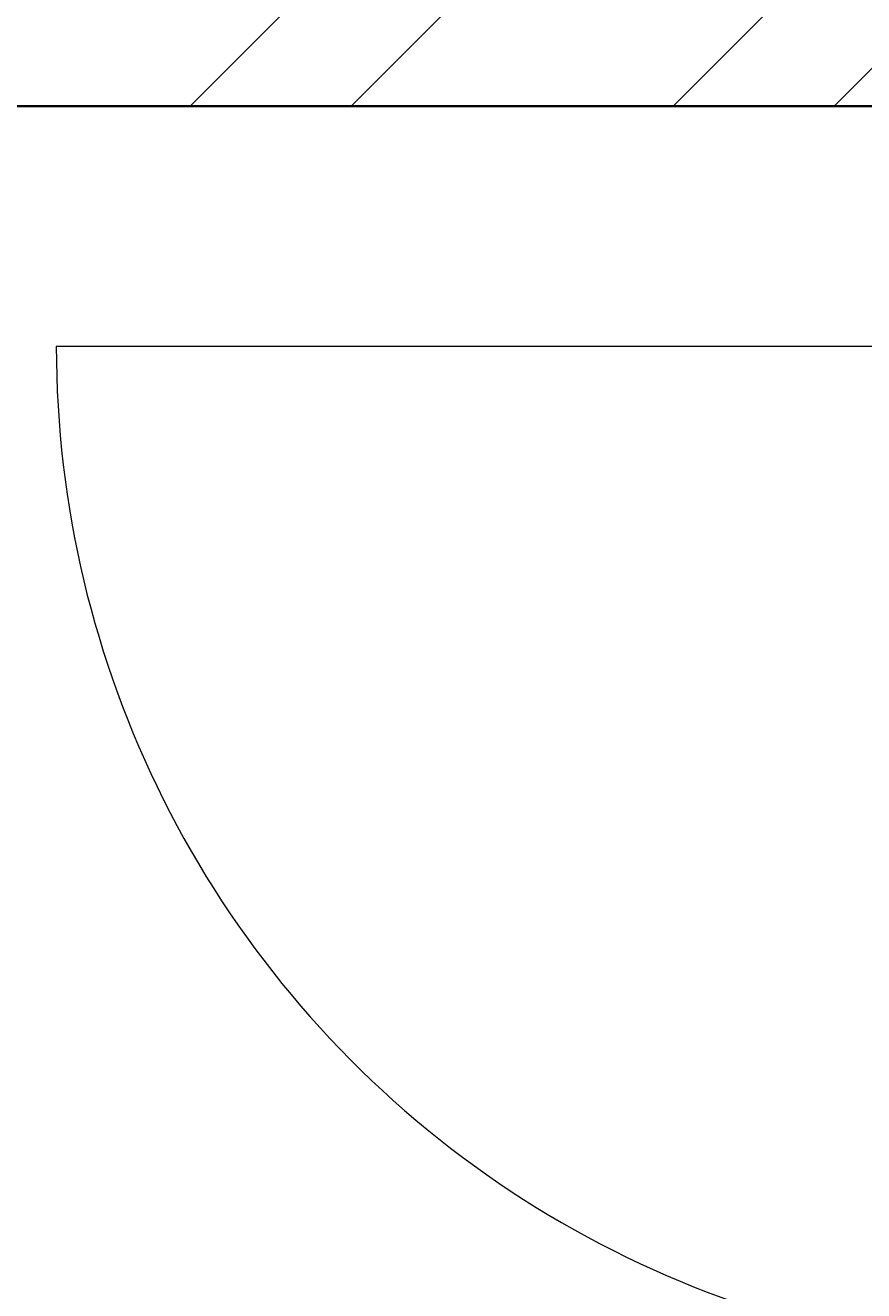
# Model space of a CAD drawing. Units: inches. Extents: x 1962 to 2771, y 1245 to 2660.
# Tile 58 of 114: x 2200 to 2224, y 2145 to 2180. Entities that reach past the tile are written whole.
import ezdxf

# ---------------------------------------------------------------- set-up
doc = ezdxf.new("R2010")
doc.units = ezdxf.units.IN
for name, color, linetype, lineweight in [('A-ANNO-DIMS', 2, 'Continuous', 18), ('A-DOOR', 3, 'Continuous', 18), ('A-WALL', 7, 'Continuous', 35), ('A-WALL-PATT', 252, 'Continuous', 13)]:
    doc.layers.add(name, color=color, linetype=linetype, lineweight=lineweight)
doc.styles.get("Standard").update_dxf_attribs({"font": 'arial.ttf'})
doc.dimstyles.get("Standard").update_dxf_attribs({"dimtxt": 0.18, "dimasz": 0.18, "dimexe": 0.18, "dimexo": 0.0625, "dimgap": 0.09, "dimtad": 0, "dimtih": 1, "dimtoh": 1, "dimdec": 4, "dimzin": 0, "dimdsep": 46, "dimtxsty": 'Standard', "dimcen": 0.09, "dimadec": 0, "dimazin": 0, "dimtfac": 1, "dimtdec": 4, "dimtofl": 0, "dimtmove": 0, "dimatfit": 3, "dimfxl": 1, "dimtolj": 1, "dimtzin": 0, "dimarcsym": 0})

# ---------------------------------------------------------------- blocks, each defined once
blk = doc.blocks.new('*D40')
at = {"layer": 'A-ANNO-DIMS', "color": 0, "lineweight": -2, "transparency": 16777216}
for p, q in [((2072.02, 2033.906), (2072.02, 2583.474)), ((2072.2, 2583.294), (2366.02, 2583.294)), ((2660.627, 2583.294), (2366.808, 2583.294)), ((2660.807, 2524.406), (2660.807, 2583.474))]:
    blk.add_line(p, q, dxfattribs=at)
at = {"layer": 'A-ANNO-DIMS', "color": 0, "transparency": 16777216}
for points in [[(2072.2, 2583.324), (2072.2, 2583.264), (2072.02, 2583.294)], [(2660.627, 2583.324), (2660.627, 2583.264), (2660.807, 2583.294)]]:
    blk.add_solid(points, dxfattribs=at)
at = {"layer": 'Defpoints', "color": 0, "transparency": 16777216}
for p in [(2660.807, 2583.294), (2660.807, 2524.344), (2072.02, 2033.844)]:
    blk.add_point(p, dxfattribs=at)
at = {"layer": 'A-ANNO-DIMS', "color": 0, "transparency": 16777216, "insert": (2366.414, 2583.294), "char_height": 0.18, "attachment_point": 5}
blk.add_mtext('\\A1;588.8', dxfattribs=at)

msp = doc.modelspace()

# ---------------------------------------------------------------- hatches: boundary and pattern name
at = {"layer": 'A-WALL-PATT'}
h = msp.add_hatch(dxfattribs=at)
h.set_pattern_fill('ANSI32', color=256)
h.paths.add_polyline_path([(2090.8074, 2467.3437), (2141.6481, 2467.3437), (2141.6481, 2469.5937), (2141.6481, 2471.8437), (2086.3074, 2471.8437), (2086.3074, 2422.5333), (2090.8074, 2422.5333)])
h.paths.add_polyline_path([(2282.7664, 2471.8437), (2204.8982, 2471.8437), (2204.8982, 2467.3437), (2234.8074, 2467.3437), (2234.8074, 2311.3437), (2228.7492, 2311.3437), (2228.7492, 2306.8437), (2234.8074, 2306.8437), (2331.9227, 2306.8437), (2331.9227, 2309.0937), (2331.9227, 2311.3437), (2239.3074, 2311.3437), (2239.3074, 2467.3437), (2282.7664, 2467.3437), (2282.7664, 2469.5937)])
h.paths.add_polyline_path([(2471.4531, 2519.8437), (2552.011, 2519.8437), (2564.3996, 2519.8437), (2564.3996, 2511.1389), (2568.8996, 2511.1389), (2568.8996, 2524.3437), (2466.9531, 2524.3437), (2466.9531, 2471.8437), (2450.0749, 2471.8437), (2446.4672, 2471.8437), (2446.4672, 2467.3437), (2450.0749, 2467.3437), (2475.9988, 2467.3437), (2475.9988, 2469.5937), (2475.9988, 2471.8437), (2471.4531, 2471.8437)])
h.paths.add_polyline_path([(2575.2231, 2469.5937), (2575.2231, 2471.8437), (2568.8996, 2471.8437), (2568.8996, 2487.1389), (2564.3996, 2487.1389), (2564.3996, 2471.8437), (2556.511, 2471.8437), (2499.2904, 2471.8437), (2499.2904, 2467.3437), (2507.8074, 2467.3437), (2507.8074, 2311.3437), (2414.863, 2311.3437), (2414.863, 2306.8437), (2512.3074, 2306.8437), (2517.0114, 2306.8437), (2517.0114, 2309.0937), (2517.0114, 2311.3437), (2512.3074, 2311.3437), (2512.3074, 2467.3437), (2575.2231, 2467.3437)])
h.paths.add_polyline_path([(2660.8074, 2471.8437), (2600.9602, 2471.8437), (2600.9602, 2467.3437), (2656.3074, 2467.3437), (2656.3074, 2432.5704), (2660.8074, 2432.5704)])
h.paths.add_polyline_path([(2660.8074, 2372.5704), (2656.3074, 2372.5704), (2656.3074, 2311.3437), (2600.276, 2311.3437), (2600.276, 2309.0937), (2600.276, 2306.8437), (2656.3074, 2306.8437), (2656.3074, 2296.2593), (2660.8074, 2296.2593)])
h.paths.add_polyline_path([(2572.3074, 2306.8437), (2577.1385, 2306.8437), (2577.1385, 2311.3437), (2551.082, 2311.3437), (2551.082, 2306.8437), (2567.8074, 2306.8437), (2567.8074, 2258.8437), (2540.0574, 2258.8437), (2540.0574, 2256.5937), (2540.0574, 2254.3437), (2567.8074, 2254.3437), (2656.3074, 2254.3437), (2656.3074, 2236.9085), (2660.8074, 2236.9085), (2660.8074, 2272.2593), (2656.3074, 2272.2593), (2656.3074, 2258.8437), (2572.3074, 2258.8437)])
h.paths.add_polyline_path([(2512.3074, 2254.3437), (2518.8716, 2254.3437), (2518.8716, 2256.5937), (2518.8716, 2258.8437), (2507.8074, 2258.8437), (2507.8074, 2177.8437), (2567.8074, 2177.8437), (2567.8074, 2172.9628), (2572.3074, 2172.9628), (2572.3074, 2177.8437), (2656.3074, 2177.8437), (2656.3074, 2166.4846), (2660.8074, 2166.4846), (2660.8074, 2200.9085), (2656.3074, 2200.9085), (2656.3074, 2182.3437), (2512.3074, 2182.3437)])
h.paths.add_polyline_path([(2656.3074, 2129.8437), (2572.3074, 2129.8437), (2572.3074, 2150.3044), (2570.0574, 2150.3044), (2567.8074, 2150.3044), (2567.8074, 2129.8437), (2507.8074, 2129.8437), (2507.8074, 2116.3027), (2510.0574, 2116.3027), (2512.3074, 2116.3027), (2512.3074, 2125.3437), (2567.8074, 2125.3437), (2572.3074, 2125.3437), (2656.3074, 2125.3437)])
h.paths.add_polyline_path([(2090.8074, 2362.5333), (2086.3074, 2362.5333), (2086.3074, 2298.6242), (2090.8074, 2298.6242), (2090.8074, 2306.8437), (2174.8074, 2306.8437), (2174.8074, 2286.4178), (2179.3074, 2286.4178), (2179.3074, 2306.8437), (2192.8641, 2306.8437), (2192.8641, 2309.0937), (2192.8641, 2311.3437), (2090.8074, 2311.3437)])
h.paths.add_polyline_path([(2209.156, 2258.8437), (2179.3074, 2258.8437), (2179.3074, 2263.2236), (2177.0574, 2263.2236), (2174.8074, 2263.2236), (2174.8074, 2258.8437), (2090.8074, 2258.8437), (2090.8074, 2274.6242), (2086.3074, 2274.6242), (2086.3074, 2238.2967), (2088.5574, 2238.2967), (2090.8074, 2238.2967), (2090.8074, 2254.3437), (2209.156, 2254.3437)])
h.paths.add_polyline_path([(2090.8074, 2177.8437), (2234.8074, 2177.8437), (2234.8074, 2173.1428), (2239.3074, 2173.1428), (2239.3074, 2258.8437), (2230.8442, 2258.8437), (2230.8442, 2256.5937), (2230.8442, 2254.3437), (2234.8074, 2254.3437), (2234.8074, 2182.3437), (2090.8074, 2182.3437), (2090.8074, 2202.2967), (2086.3074, 2202.2967), (2086.3074, 2140.0389), (2090.8074, 2140.0389)])
h.paths.add_polyline_path([(2090.8074, 2080.0389), (2086.3074, 2080.0389), (2086.3074, 2033.8437), (2090.8074, 2033.8437)], flags=17)
h.paths.add_polyline_path([(2244.9405, 2033.8437), (2239.3074, 2033.8437), (2239.3074, 2142.0665), (2237.2592, 2142.0665), (2234.8074, 2142.0665), (2234.8074, 2033.8437), (2090.8074, 2033.8437), (2076.5204, 2033.8437), (2072.0204, 2033.8437), (2072.0204, 2000.4493), (2076.5204, 2000.4493), (2076.5204, 2029.3437), (2090.8074, 2029.3437), (2244.9405, 2029.3437), (2244.9405, 2031.5937)])
h.paths.add_polyline_path([(2234.8074, 1933.3437), (2076.5204, 1933.3437), (2076.5204, 1952.4493), (2074.2704, 1952.4493), (2072.0204, 1952.4493), (2072.0204, 1933.3437), (2072.0204, 1928.8437), (2234.8074, 1928.8437)])
h.paths.add_polyline_path([(2090.8074, 1928.8437), (2086.3074, 1928.8437), (2086.3074, 1906.5013), (2090.8074, 1906.5013)])
h.paths.add_polyline_path([(2090.8074, 1846.5013), (2086.3074, 1846.5013), (2086.3074, 1769.9917), (2088.5574, 1769.9917), (2090.8074, 1769.9917), (2090.8074, 1780.3437), (2234.8074, 1780.3437), (2234.8074, 1708.3437), (2230.3764, 1708.3437), (2230.3764, 1703.8437), (2239.3074, 1703.8437), (2239.3074, 1792.6669), (2237.0574, 1792.6669), (2234.8074, 1792.6669), (2234.8074, 1784.8437), (2090.8074, 1784.8437)])
h.paths.add_polyline_path([(2239.3074, 1928.8437), (2244.9405, 1928.8437), (2244.9405, 1931.0937), (2244.9405, 1933.3437), (2234.8074, 1933.3437), (2234.8074, 1928.8437), (2234.8074, 1825.5949), (2239.3074, 1825.5949)])
h.paths.add_polyline_path([(2148.0425, 1649.0937), (2148.0425, 1651.3437), (2090.8074, 1651.3437), (2090.8074, 1646.8437), (2148.0425, 1646.8437)], flags=0)
h.paths.add_polyline_path([(2207.5601, 1708.3437), (2090.8074, 1708.3437), (2090.8074, 1703.8437), (2174.8074, 1703.8437), (2174.8074, 1651.3437), (2170.4457, 1651.3437), (2170.4457, 1646.8437), (2195.9924, 1646.8437), (2195.9924, 1649.0937), (2195.9924, 1651.3437), (2179.3074, 1651.3437), (2179.3074, 1703.8437), (2207.5601, 1703.8437), (2207.5601, 1706.0937)])
h.paths.add_polyline_path([(2090.8074, 1733.9917), (2086.3074, 1733.9917), (2086.3074, 1696.1032), (2088.5574, 1696.1032), (2090.8074, 1696.1032)])
h.paths.add_polyline_path([(2090.8074, 1672.1032), (2086.3074, 1672.1032), (2086.3074, 1600.3335), (2090.8074, 1600.3335)])
h.paths.add_polyline_path([(2090.8074, 1540.3335), (2086.3074, 1540.3335), (2086.3074, 1486.3437), (2139.6766, 1486.3437), (2139.6766, 1490.8437), (2090.8074, 1490.8437)])
h.paths.add_polyline_path([(2302.3876, 1490.8437), (2239.3074, 1490.8437), (2239.3074, 1646.8437), (2335.9994, 1646.8437), (2335.9994, 1651.3437), (2229.884, 1651.3437), (2229.884, 1646.8437), (2234.8074, 1646.8437), (2234.8074, 1490.8437), (2202.7103, 1490.8437), (2202.7103, 1488.5937), (2202.7103, 1486.3437), (2275.0699, 1486.3437), (2275.0699, 1475.772), (2279.5699, 1475.772), (2279.5699, 1486.3437), (2302.3876, 1486.3437)])
h.paths.add_polyline_path([(2279.5699, 1451.772), (2275.0699, 1451.772), (2275.0699, 1438.3437), (2174.8074, 1438.3437), (2174.8074, 1486.3437), (2179.7922, 1486.3437), (2179.7922, 1490.8437), (2163.3585, 1490.8437), (2163.3585, 1488.5937), (2163.3585, 1486.3437), (2170.3074, 1486.3437), (2170.3074, 1433.8437), (2279.5699, 1433.8437)])
h.paths.add_polyline_path([(2427.2363, 1490.8437), (2375.8074, 1490.8437), (2375.8074, 1646.8437), (2381.6401, 1646.8437), (2381.6401, 1651.3437), (2365.887, 1651.3437), (2365.887, 1649.0937), (2365.887, 1646.8437), (2371.3074, 1646.8437), (2371.3074, 1490.8437), (2327.5627, 1490.8437), (2327.5627, 1488.5937), (2327.5627, 1486.3437), (2371.3074, 1486.3437), (2371.3074, 1433.8437), (2375.8074, 1433.8437), (2375.8074, 1486.3437), (2427.2363, 1486.3437)])
h.paths.add_polyline_path([(2512.3074, 1646.8437), (2519.4351, 1646.8437), (2519.4351, 1649.0937), (2519.4351, 1651.3437), (2507.8074, 1651.3437), (2416.0063, 1651.3437), (2416.0063, 1649.0937), (2416.0063, 1646.8437), (2507.8074, 1646.8437), (2507.8074, 1490.8437), (2497.0532, 1490.8437), (2497.0532, 1488.5937), (2497.0532, 1486.3437), (2574.9344, 1486.3437), (2574.9344, 1476.0181), (2579.4344, 1476.0181), (2579.4344, 1486.3437), (2584.4872, 1486.3437), (2584.3074, 1490.8437), (2512.3074, 1490.8437)])
h.paths.add_polyline_path([(2470.5091, 1486.3437), (2473.9767, 1486.3437), (2473.9767, 1490.8437), (2449.6605, 1490.8437), (2449.6605, 1488.5937), (2449.6605, 1486.3437), (2466.0091, 1486.3437), (2466.0091, 1433.8437), (2470.5091, 1433.8437), (2579.4344, 1433.8437), (2579.4344, 1452.0181), (2574.9344, 1452.0181), (2574.9344, 1438.3437), (2554.5091, 1438.3437), (2470.5091, 1438.3437)])
h.paths.add_polyline_path([(2656.3074, 1490.8437), (2611.86, 1490.8437), (2611.86, 1486.3437), (2656.3074, 1486.3437)])
h.paths.add_polyline_path([(2660.8074, 1532.7007), (2658.5574, 1532.7007), (2656.3074, 1532.7007), (2656.3074, 1486.3437), (2660.8074, 1486.3437)])
h.paths.add_polyline_path([(2660.8074, 1664.9663), (2656.3074, 1664.9663), (2656.3074, 1651.3437), (2602.2313, 1651.3437), (2602.2313, 1646.8437), (2656.3074, 1646.8437), (2656.3074, 1592.7007), (2660.8074, 1592.7007)])
h.paths.add_polyline_path([(2660.8074, 1724.5221), (2656.3074, 1724.5221), (2656.3074, 1703.8437), (2542.4725, 1703.8437), (2542.4725, 1699.3437), (2567.8074, 1699.3437), (2567.8074, 1651.3437), (2552.7766, 1651.3437), (2552.7766, 1649.0937), (2552.7766, 1646.8437), (2577.2878, 1646.8437), (2577.2878, 1649.0937), (2577.2878, 1651.3437), (2572.3074, 1651.3437), (2572.3074, 1699.3437), (2656.3074, 1699.3437), (2656.3074, 1688.9663), (2660.8074, 1688.9663)])
h.paths.add_polyline_path([(2660.8074, 1880.6524), (2656.3074, 1880.6524), (2656.3074, 1832.8437), (2512.3074, 1832.8437), (2512.3074, 1837.8959), (2507.8074, 1837.8959), (2507.8074, 1828.3437), (2567.8074, 1828.3437), (2567.8074, 1804.3437), (2572.3074, 1804.3437), (2572.3074, 1828.3437), (2656.3074, 1828.3437), (2656.3074, 1818.6778), (2660.8074, 1818.6778)])
h.paths.add_polyline_path([(2660.8074, 1794.6778), (2656.3074, 1794.6778), (2656.3074, 1780.3437), (2572.3074, 1780.3437), (2572.3074, 1783.0303), (2570.0574, 1783.0303), (2567.8074, 1783.0303), (2567.8074, 1780.3437), (2507.8074, 1780.3437), (2507.8074, 1699.3437), (2517.8858, 1699.3437), (2517.8858, 1701.5937), (2517.8858, 1703.8437), (2512.3074, 1703.8437), (2512.3074, 1775.8437), (2656.3074, 1775.8437), (2656.3074, 1760.5221), (2660.8074, 1760.5221)])
h.paths.add_polyline_path([(2660.8074, 1981.3437), (2660.8074, 2020.2808), (2658.5574, 2020.2808), (2656.3074, 2020.2808), (2656.3074, 1981.3437), (2512.3074, 1981.3437), (2512.3074, 2086.6996), (2507.8074, 2086.6996), (2507.8074, 1981.3437), (2375.8074, 1981.3437), (2375.8074, 1986.8505), (2373.5574, 1986.8505), (2371.3074, 1986.8505), (2371.3074, 1973.2607), (2375.8074, 1973.2607), (2375.8074, 1976.8437), (2507.8074, 1976.8437), (2507.8074, 1865.4281), (2510.0574, 1865.4281), (2512.3074, 1865.4281), (2512.3074, 1976.8437), (2660.8074, 1976.8437)])
h.paths.add_polyline_path([(2375.8074, 1940.297), (2373.5574, 1940.297), (2371.3074, 1940.297), (2371.3074, 1933.3437), (2278.4434, 1933.3437), (2278.4434, 1928.8437), (2371.3074, 1928.8437), (2371.3074, 1651.3437), (2375.8074, 1651.3437)])
h.paths.add_polyline_path([(2660.8074, 1976.8437), (2656.3074, 1976.8437), (2656.3074, 1940.6524), (2660.8074, 1940.6524)], flags=17)
h.paths.add_polyline_path([(2660.8074, 2142.4846), (2656.3074, 2142.4846), (2656.3074, 2080.2808), (2660.8074, 2080.2808)])
h.paths.add_polyline_path([(2381.4189, 2311.3437), (2375.8074, 2311.3437), (2375.8074, 2467.3437), (2424.7242, 2467.3437), (2424.7242, 2469.5937), (2424.7242, 2471.8437), (2375.8074, 2471.8437), (2375.8074, 2524.3437), (2371.3074, 2524.3437), (2371.3074, 2471.8437), (2307.2097, 2471.8437), (2307.2097, 2467.3437), (2371.3074, 2467.3437), (2371.3074, 2311.3437), (2366.8901, 2311.3437), (2366.8901, 2306.8437), (2371.3074, 2306.8437), (2371.3074, 2033.8437), (2279.6589, 2033.8437), (2279.6589, 2029.3437), (2371.3074, 2029.3437), (2371.3074, 2014.2598), (2375.8074, 2014.2598), (2375.8074, 2306.8437), (2381.4189, 2306.8437)])
h.paths.add_polyline_path([(2263.3074, 2524.3437), (2170.3074, 2524.3437), (2170.3074, 2519.8437), (2170.3074, 2471.8437), (2165.0312, 2471.8437), (2165.0312, 2467.3437), (2179.6721, 2467.3437), (2179.6721, 2469.5161), (2179.6721, 2471.8437), (2174.8074, 2471.8437), (2174.8074, 2519.8437), (2258.8074, 2519.8437), (2258.8074, 2511.6436), (2263.3074, 2511.6436)])
h.paths.add_polyline_path([(2245.0232, 1361.4123), (2492.9468, 1361.4123), (2492.9468, 1398.505), (2245.0232, 1398.505)], flags=9)
h.paths.add_polyline_path([(2388.1434, 2086.6936), (2425.0704, 2086.6936), (2425.0704, 2105.3509), (2388.1434, 2105.3509)], flags=9)
h.paths.add_polyline_path([(2404.922, 2242.6744), (2445.7337, 2242.6744), (2445.7337, 2261.3318), (2404.922, 2261.3318)], flags=9)
h.paths.add_polyline_path([(2269.4107, 2156.7935), (2306.3378, 2156.7935), (2306.3378, 2175.4508), (2269.4107, 2175.4508)], flags=9)
h.paths.add_polyline_path([(2269.3277, 2233.4343), (2306.2547, 2233.4343), (2306.2547, 2252.0917), (2269.3277, 2252.0917)], flags=9)
h.paths.add_polyline_path([(2431.6052, 2320.6922), (2470.4456, 2320.6922), (2470.4456, 2339.3495), (2431.6052, 2339.3495)], flags=25)
h.paths.add_polyline_path([(2249.6902, 2315.7608), (2288.5306, 2315.7608), (2288.5306, 2334.4182), (2249.6902, 2334.4182)], flags=25)
h.paths.add_polyline_path([(2096.9301, 2314.3181), (2135.7704, 2314.3181), (2135.7704, 2332.9755), (2096.9301, 2332.9755)], flags=25)
h.paths.add_polyline_path([(2134.3475, 2285.7089), (2161.4655, 2285.7089), (2161.4655, 2304.3662), (2134.3475, 2304.3662)], flags=9)
h.paths.add_polyline_path([(2126.5155, 2209.4076), (2159.9227, 2209.4076), (2159.9227, 2228.065), (2126.5155, 2228.065)], flags=25)
h.paths.add_polyline_path([(2110.5753, 2141.5299), (2149.4157, 2141.5299), (2149.4157, 2160.1872), (2110.5753, 2160.1872)], flags=25)
h.paths.add_polyline_path([(2249.8618, 1968.3317), (2286.3966, 1968.3317), (2286.3966, 1986.989), (2249.8618, 1986.989)], flags=9)
h.paths.add_polyline_path([(2395.9507, 1777.0051), (2436.7624, 1777.0051), (2436.7624, 1795.6625), (2395.9507, 1795.6625)], flags=9)
h.paths.add_polyline_path([(2398.5259, 1888.5651), (2435.0062, 1888.5651), (2435.0062, 1907.2224), (2398.5259, 1907.2224)], flags=25)
h.paths.add_polyline_path([(2259.3506, 1728.3559), (2296.2776, 1728.3559), (2296.2776, 1747.0132), (2259.3506, 1747.0132)], flags=9)
h.paths.add_polyline_path([(2271.3698, 1845.268), (2308.2968, 1845.268), (2308.2968, 1863.9253), (2271.3698, 1863.9253)], flags=9)
h.paths.add_polyline_path([(2120.9355, 1786.3027), (2159.7759, 1786.3027), (2159.7759, 1804.9601), (2120.9355, 1804.9601)], flags=25)
h.paths.add_polyline_path([(2121.3164, 1732.1043), (2154.7236, 1732.1043), (2154.7236, 1750.7616), (2121.3164, 1750.7616)], flags=25)
h.paths.add_polyline_path([(2118.3706, 1678.8997), (2147.5282, 1678.8997), (2147.5282, 1697.557), (2118.3706, 1697.557)], flags=25)
h.paths.add_polyline_path([(2385.9227, 1493.557), (2424.763, 1493.557), (2424.763, 1512.2143), (2385.9227, 1512.2143)], flags=25)
h.paths.add_polyline_path([(2248.7058, 1500.0256), (2287.5462, 1500.0256), (2287.5462, 1518.6829), (2248.7058, 1518.6829)], flags=25)
h.paths.add_polyline_path([(2104.1669, 1617.3771), (2143.0073, 1617.3771), (2143.0073, 1636.0344), (2104.1669, 1636.0344)], flags=9)
h.paths.add_polyline_path([(2096.0714, 1447.8824), (2137.3845, 1447.8824), (2137.3845, 1458.1859), (2096.0714, 1458.1859)], flags=9)
h.paths.add_polyline_path([(2180.6114, 1440.325), (2209.7689, 1440.325), (2209.7689, 1458.9823), (2180.6114, 1458.9823)], flags=25)
h.paths.add_polyline_path([(2316.1698, 1447.9637), (2357.4829, 1447.9637), (2357.4829, 1458.2673), (2316.1698, 1458.2673)], flags=9)
h.paths.add_polyline_path([(2397.6187, 1447.9637), (2438.9318, 1447.9637), (2438.9318, 1458.2673), (2397.6187, 1458.2673)], flags=9)
h.paths.add_polyline_path([(2473.0778, 1439.5953), (2502.2354, 1439.5953), (2502.2354, 1458.2527), (2473.0778, 1458.2527)], flags=25)
h.paths.add_polyline_path([(2589.7027, 1447.8819), (2631.0158, 1447.8819), (2631.0158, 1458.1855), (2589.7027, 1458.1855)], flags=9)
h.paths.add_polyline_path([(2522.4009, 1497.5285), (2561.2413, 1497.5285), (2561.2413, 1516.1859), (2522.4009, 1516.1859)], flags=25)
h.paths.add_polyline_path([(2579.6565, 1671.3482), (2608.8141, 1671.3482), (2608.8141, 1690.0056), (2579.6565, 1690.0056)], flags=25)
h.paths.add_polyline_path([(2544.7038, 1725.5064), (2578.1111, 1725.5064), (2578.1111, 1744.1637), (2544.7038, 1744.1637)], flags=25)
h.paths.add_polyline_path([(2578.1191, 1807.472), (2607.2766, 1807.472), (2607.2766, 1826.1293), (2578.1191, 1826.1293)], flags=25)
h.paths.add_polyline_path([(2595.0614, 1835.1839), (2633.9018, 1835.1839), (2633.9018, 1853.8413), (2595.0614, 1853.8413)], flags=25)
h.paths.add_polyline_path([(2567.0097, 2097.7035), (2605.8501, 2097.7035), (2605.8501, 2116.3609), (2567.0097, 2116.3609)], flags=9)
h.paths.add_polyline_path([(2586.644, 2134.6454), (2615.8015, 2134.6454), (2615.8015, 2153.3027), (2586.644, 2153.3027)], flags=9)
h.paths.add_polyline_path([(2544.6185, 2212.6783), (2578.0258, 2212.6783), (2578.0258, 2231.3356), (2544.6185, 2231.3356)], flags=25)
h.paths.add_polyline_path([(2577.0273, 2256.9023), (2606.1849, 2256.9023), (2606.1849, 2275.5597), (2577.0273, 2275.5597)], flags=24)
h.paths.add_polyline_path([(2605.2683, 2315.2821), (2644.1087, 2315.2821), (2644.1087, 2333.9395), (2605.2683, 2333.9395)], flags=25)
h.paths.add_polyline_path([(2583.1244, 2496.1815), (2624.4375, 2496.1815), (2624.4375, 2506.4851), (2583.1244, 2506.4851)], flags=9)
h.paths.add_polyline_path([(2474.761, 2497.0823), (2503.9185, 2497.0823), (2503.9185, 2515.7397), (2474.761, 2515.7397)], flags=25)
h.paths.add_polyline_path([(2387.5787, 2494.2563), (2428.902, 2494.2563), (2428.902, 2504.5598), (2387.5787, 2504.5598)], flags=9)
h.paths.add_polyline_path([(2300.1657, 2500.1564), (2341.4788, 2500.1564), (2341.4788, 2510.46), (2300.1657, 2510.46)], flags=25)
h.paths.add_polyline_path([(2176.8589, 2497.5843), (2206.0165, 2497.5843), (2206.0165, 2516.2416), (2176.8589, 2516.2416)], flags=25)
h.paths.add_polyline_path([(2097.4668, 2494.9762), (2138.7799, 2494.9762), (2138.7799, 2505.2798), (2097.4668, 2505.2798)], flags=9)

# ---------------------------------------------------------------- linework, layer by layer
at = {"layer": 'A-DOOR'}
msp.add_line((2237.0574, 2171.1428), (2201.0574, 2171.1428), dxfattribs=at)
msp.add_arc((2229.2838, 2171.1428), 28.2264, 180, 286.41252, dxfattribs=at)
at = {"layer": 'A-WALL'}
msp.add_line((2090.8074, 2177.8437), (2234.8074, 2177.8437), dxfattribs=at)

# ---------------------------------------------------------------- dimensions: what is measured, and where the dimension line sits
at = {"layer": 'A-ANNO-DIMS'}
dim = msp.add_linear_dim(base=(2660.8074, 2583.2937), p1=(2072.0204, 2033.8437), p2=(2660.8074, 2524.3437), dimstyle='Standard', override={"dimdec": 1, "dimlfac": 1, "dimrnd": 0, "dimzin": 0, "dimdsep": 46, "dimlunit": 2}, dxfattribs=at)
dim.commit()
dim.dimension.update_dxf_attribs({"geometry": '*D40', "text_midpoint": (2366.4139, 2583.2937)})

doc.saveas('drawing.dxf')
